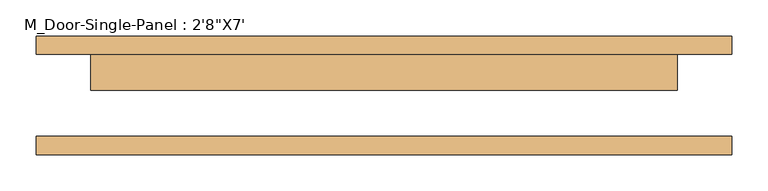
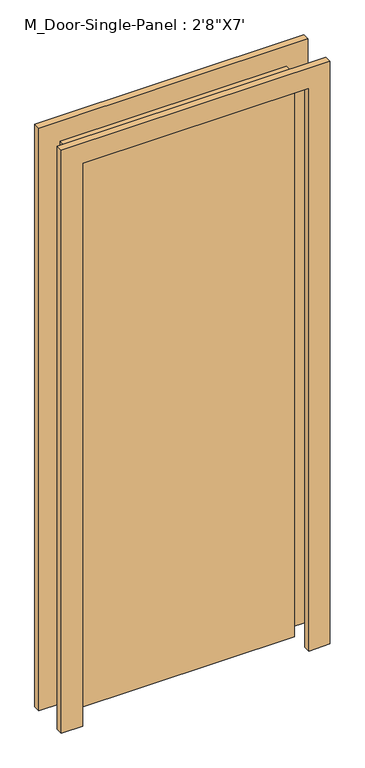
"""IFC4 building model written with IfcOpenShell, lengths in millimetres: door geometry."""

from ifc_helpers import new_model, si_unit, frame, origin, origin_with_axes, place, context, project, spatial, polyline, outline, extrude, source, transform, mapped, element, save


def door_4c0a2014(model_context):
    return source(origin(), model_context, "Body", "SweptSolid", [
        extrude(outline(polyline([(406.4, 7.15), (-406.4, 7.15), (-406.4, 57.15), (406.4, 57.15), (406.4, 7.15)])), origin_with_axes(), (0.0, 0.0, 1.0), 2133.6),
        extrude(outline(polyline([(2209.8, 482.6), (2209.8, -482.6), (0.0, -482.6), (0.0, -406.4), (2133.6, -406.4), (2133.6, 406.4), (0.0, 406.4), (0.0, 482.6), (2209.8, 482.6)])), frame((0.0, -82.15, 0.0), z_axis=(0.0, 1.0, 0.0), x_axis=(0.0, 0.0, 1.0)), (0.0, 0.0, 1.0), 25.0),
        extrude(outline(polyline([(2209.8, -482.6), (0.0, -482.6), (0.0, -406.4), (2133.6, -406.4), (2133.6, 406.4), (0.0, 406.4), (0.0, 482.6), (2209.8, 482.6), (2209.8, -482.6)])), frame((0.0, 57.15, 0.0), z_axis=(0.0, 1.0, 0.0), x_axis=(0.0, 0.0, 1.0)), (0.0, 0.0, 1.0), 25.0),
    ])


if __name__ == "__main__":
    model = new_model("IFC4")
    model_context = context("Model", 3, world=origin())
    ifc_project = project(units=[si_unit("LENGTHUNIT", "METRE", prefix="MILLI")], contexts=[model_context])
    site = spatial("IfcSite", under=ifc_project)
    building = spatial("IfcBuilding", under=site)
    placement = place(None, origin())
    door_shape = door_4c0a2014(model_context)
    element("IfcDoor", 1, ObjectType="M_Door-Single-Panel : 2'8\"X7'", at=placement, inside=building, context=model_context, shape_type="MappedRepresentation", body=[
        mapped(door_shape, transform((0.0, 0.0, 0.0), x_axis=(1.0, 0.0, 0.0), y_axis=(0.0, 1.0, 0.0), z_axis=(0.0, 0.0, 1.0))),
    ])
    save(model, "model.ifc")

# Revit data of these elements
# Type "M_Door-Single-Panel : 2'8\"X7'"
#   Type Mark = "9"
#   Construction Type Id = "DOOR"
#   Assembly Code = "C1020300"
#   Analytic Construction = "Wooden"
#   Thickness = 0' - 1.9685"
#   Thermal Resistance (R) = 2.5876 (h·ft²·°F)/BTU
#   Swing Angle [instance default] = 90.00°
#   Heat Transfer Coefficient (U) = 0.3865 BTU/(h·ft²·°F)
#   Height = 7' - 0"
#   Trim Projection Ext = 0' - 0.98425"
#   Trim Projection Int = 0' - 0.98425"
#   Trim Width = 0' - 3.14961"
#   Width = 2' - 8"
#   Define Thermal Properties by = 1
#   Panel Material = Wood - Birch - Solid Stained Light Low Gloss
#   Trim Material = Paint - Sienna
#   Visual Light Transmittance = 0
#   Solar Heat Gain Coefficient = 0
#   Function = (empty or 0)
#   Wall Closure = (empty or 0)
# Element 1 (IfcDoor, "M_Door-Single-Panel : 2'8\"X7'")
#   Materials on its faces: "Paint - Sienna", "Wood - Birch - Solid Stained Light Low Gloss"
# Materials
#   "Wood - Birch - Solid Stained Light Low Gloss": class "Wood", colour RGB 210 159 95, transparency 0, Cost = 0
#   "Paint - Sienna": colour RGB 118 70 51, transparency 0, Cost = 0
